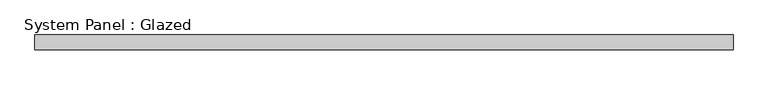
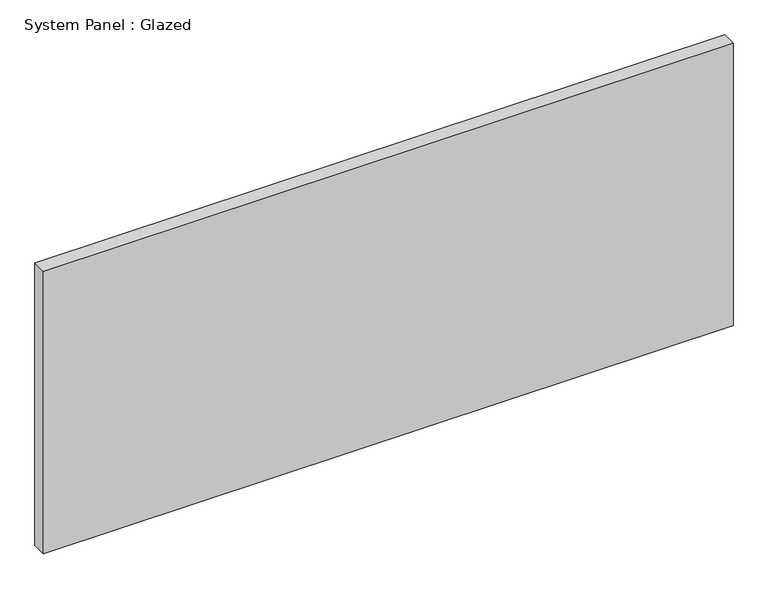
"""IFC4 building model written with IfcOpenShell, lengths in millimetres: plate geometry, System Panel : Glazed."""

from ifc_helpers import new_model, si_unit, origin, origin_with_axes, place, context, project, spatial, polyline, outline, extrude, source, transform, mapped, element, save


def system_panel_glazed_1bdee89b(model_context):
    return source(origin(), model_context, "Body", "SweptSolid", [
        extrude(outline(polyline([(593.7250001, -44.45), (-593.7250001, -44.45), (-593.7250001, -19.05), (593.7250001, -19.05), (593.7250001, -44.45)])), origin_with_axes(), (0.0, 0.0, 1.0), 514.35),
    ])


if __name__ == "__main__":
    model = new_model("IFC4")
    model_context = context("Model", 3, world=origin())
    ifc_project = project(units=[si_unit("LENGTHUNIT", "METRE", prefix="MILLI")], contexts=[model_context])
    site = spatial("IfcSite", under=ifc_project)
    building = spatial("IfcBuilding", under=site)
    placement = place(None, origin())
    system_panel_glazed_shape = system_panel_glazed_1bdee89b(model_context)
    element("IfcPlate", 1, ObjectType="System Panel : Glazed", at=placement, inside=building, context=model_context, shape_type="MappedRepresentation", body=[
        mapped(system_panel_glazed_shape, transform((0.0, 0.0, 0.0), x_axis=(1.0, 0.0, 0.0), y_axis=(0.0, 1.0, 0.0), z_axis=(0.0, 0.0, 1.0))),
    ])
    save(model, "model.ifc")

# Revit data of these elements
# Type "System Panel : Glazed"
#   Construction Type Id = "GSP4R"
#   Analytic Construction = "1/8 in Pilkington single glazing"
#   Visual Light Transmittance = 0.9
#   Solar Heat Gain Coefficient = 0.86
#   Heat Transfer Coefficient (U) = 1.18115 BTU/(h·ft²·°F)
#   Define Thermal Properties by = 1
# Element 1 (IfcPlate, "System Panel : Glazed")
#   Materials on its faces: "glass panel 223"
# Materials
#   "glass panel 223": class "Generic", colour RGB 120 120 120, transparency 0, Cost = 0
